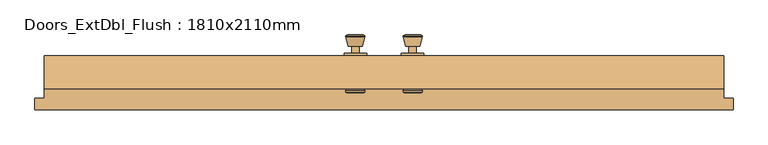
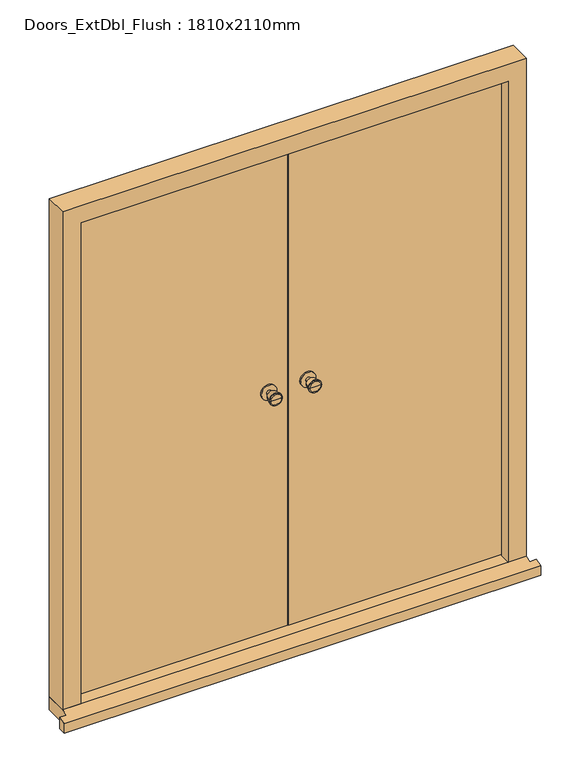
"""IFC4 building model written with IfcOpenShell, lengths in millimetres: door geometry, Doors_ExtDbl_Flush : 1810x2110mm."""

from ifc_helpers import new_model, si_unit, point, frame, frame_2d, origin, place, context, project, spatial, polyline, circle_curve, trimmed, segment, composite_curve, outline, extrude, faceted_brep, source, transform, mapped, element, save
from ifc_brep_helpers import plane_surface, cylinder_surface, revolved_surface, advanced_brep


def doors_extdbl_flush_1810x2110mm_cf8af4c5(model_context):
    return source(origin(), model_context, "Body", "SolidModel", [
        advanced_brep(
        [(-76.5, 7.5, 1050.0), (-86.5, 7.5, 1050.0), (-66.5, 7.5, 1050.0), (-96.9758676, 56.5, 1050.0), (-76.5, 56.5, 1050.0), (-56.0241324, 56.5, 1050.0), (-101.5, 54.6721319, 1050.0), (-51.5, 54.6721319, 1050.0), (-101.5, 51.2084537, 1050.0), (-51.5, 51.2084537, 1050.0), (-95.136236, 26.5, 1050.0), (-57.863764, 26.5, 1050.0), (-86.5, 26.5, 1050.0), (-66.5, 26.5, 1050.0)],
        [
            (0, 1),
            (1, 2, circle_curve(frame((-76.5, 7.5, 1050.0), z_axis=(0.0, -1.0, 0.0), x_axis=(1.0, 0.0, 0.0)), 10.0)),
            (2, 0),
            (2, 1, circle_curve(frame((-76.5, 7.5, 1050.0), z_axis=(0.0, -1.0, 0.0), x_axis=(1.0, 0.0, 0.0)), 10.0)),
            (3, 4),
            (4, 5),
            (5, 3, circle_curve(frame((-76.5, 56.5, 1050.0), z_axis=(0.0, 1.0, 0.0), x_axis=(1.0, 0.0, 0.0)), 20.4758676)),
            (3, 5, circle_curve(frame((-76.5, 56.5, 1050.0), z_axis=(0.0, 1.0, 0.0), x_axis=(1.0, 0.0, 0.0)), 20.4758676)),
            (6, 3),
            (5, 7),
            (7, 6, circle_curve(frame((-76.5, 54.6721319, 1050.0), z_axis=(0.0, 1.0, 0.0), x_axis=(1.0, 0.0, 0.0)), 25.0)),
            (6, 7, circle_curve(frame((-76.5, 54.6721319, 1050.0), z_axis=(0.0, 1.0, 0.0), x_axis=(1.0, 0.0, 0.0)), 25.0)),
            (8, 6),
            (7, 9),
            (9, 8, circle_curve(frame((-76.5, 51.2084537, 1050.0), z_axis=(0.0, 1.0, 0.0), x_axis=(1.0, 0.0, 0.0)), 25.0)),
            (8, 9, circle_curve(frame((-76.5, 51.2084537, 1050.0), z_axis=(0.0, 1.0, 0.0), x_axis=(1.0, 0.0, 0.0)), 25.0)),
            (10, 8),
            (9, 11),
            (11, 10, circle_curve(frame((-76.5, 26.5, 1050.0), z_axis=(0.0, 1.0, 0.0), x_axis=(1.0, 0.0, 0.0)), 18.636236)),
            (10, 11, circle_curve(frame((-76.5, 26.5, 1050.0), z_axis=(0.0, 1.0, 0.0), x_axis=(1.0, 0.0, 0.0)), 18.636236)),
            (12, 10),
            (11, 13),
            (13, 12, circle_curve(frame((-76.5, 26.5, 1050.0), z_axis=(0.0, 1.0, 0.0), x_axis=(1.0, 0.0, 0.0)), 10.0)),
            (12, 13, circle_curve(frame((-76.5, 26.5, 1050.0), z_axis=(0.0, 1.0, 0.0), x_axis=(1.0, 0.0, 0.0)), 10.0)),
            (1, 12),
            (13, 2),
        ],
        [
            plane_surface(frame((-76.5, 7.5, 1050.0), z_axis=(0.0, -1.0, 0.0), x_axis=(1.0, 0.0, 0.0))),
            plane_surface(frame((-76.5, 56.5, 1050.0), z_axis=(0.0, 1.0, 0.0), x_axis=(1.0, 0.0, 0.0))),
            revolved_surface(polyline([(-56.0241324, 56.5, 1050.0), (-51.5, 54.6721319, 1050.0)]), (-76.5, 7.5, 1050.0), (0.0, -1.0, 0.0)),
            cylinder_surface(frame((-76.5, 7.5, 1050.0), z_axis=(0.0, -1.0, 0.0), x_axis=(1.0, 0.0, 0.0)), 25.0),
            revolved_surface(polyline([(-51.5, 51.2084537, 1050.0), (-57.863764, 26.5, 1050.0)]), (-76.5, 7.5, 1050.0), (0.0, -1.0, 0.0)),
            plane_surface(frame((-76.5, 26.5, 1050.0), z_axis=(0.0, -1.0, 0.0), x_axis=(1.0, 0.0, 0.0))),
            cylinder_surface(frame((-76.5, 7.5, 1050.0), z_axis=(0.0, -1.0, 0.0), x_axis=(1.0, 0.0, 0.0)), 10.0),
        ],
        [
            (0, [[1, 2, 3]]),
            (0, [[-3, 4, -1]]),
            (1, [[5, 6, 7]]),
            (1, [[-6, -5, 8]]),
            (2, [[9, -7, 10, 11]]),
            (2, [[-10, -8, -9, 12]]),
            (3, [[13, -11, 14, 15]]),
            (3, [[-14, -12, -13, 16]]),
            (4, [[17, -15, 18, 19]]),
            (4, [[-18, -16, -17, 20]]),
            (5, [[21, -19, 22, 23]]),
            (5, [[-22, -20, -21, 24]]),
            (6, [[25, -23, 26, -2]]),
            (6, [[-26, -24, -25, -4]]),
        ],
    ),
        extrude(outline(composite_curve([segment(trimmed(circle_curve(frame_2d((1050.0, -76.5)), 30.0), [point((1050.0, -46.5))], [point((1050.0, -106.5))], False, "CARTESIAN"), True, "CONTINUOUS"), segment(trimmed(circle_curve(frame_2d((1050.0, -76.5)), 30.0), [point((1050.0, -106.5))], [point((1050.0, -46.5))], False, "CARTESIAN"), True, "CONTINUOUS")], self_intersect=False)), frame((0.0, 1.5, 0.0), z_axis=(0.0, 1.0, 0.0), x_axis=(0.0, 0.0, 1.0)), (0.0, 0.0, 1.0), 6.0),
        advanced_brep(
        [(-76.5, -48.5, 1050.0), (-66.5, -48.5, 1050.0), (-86.5, -48.5, 1050.0), (-96.9758676, -97.5, 1050.0), (-56.0241324, -97.5, 1050.0), (-76.5, -97.5, 1050.0), (-101.5, -95.6721319, 1050.0), (-51.5, -95.6721319, 1050.0), (-101.5, -92.2084537, 1050.0), (-51.5, -92.2084537, 1050.0), (-95.136236, -67.5, 1050.0), (-57.863764, -67.5, 1050.0), (-86.5, -67.5, 1050.0), (-66.5, -67.5, 1050.0)],
        [
            (0, 1),
            (1, 2, circle_curve(frame((-76.5, -48.5, 1050.0), z_axis=(0.0, 1.0, 0.0), x_axis=(1.0, 0.0, 0.0)), 10.0)),
            (2, 0),
            (2, 1, circle_curve(frame((-76.5, -48.5, 1050.0), z_axis=(0.0, 1.0, 0.0), x_axis=(1.0, 0.0, 0.0)), 10.0)),
            (3, 4, circle_curve(frame((-76.5, -97.5, 1050.0), z_axis=(0.0, -1.0, 0.0), x_axis=(1.0, 0.0, 0.0)), 20.4758676)),
            (4, 5),
            (5, 3),
            (4, 3, circle_curve(frame((-76.5, -97.5, 1050.0), z_axis=(0.0, -1.0, 0.0), x_axis=(1.0, 0.0, 0.0)), 20.4758676)),
            (6, 7, circle_curve(frame((-76.5, -95.6721319, 1050.0), z_axis=(0.0, -1.0, 0.0), x_axis=(1.0, 0.0, 0.0)), 25.0)),
            (7, 4),
            (3, 6),
            (7, 6, circle_curve(frame((-76.5, -95.6721319, 1050.0), z_axis=(0.0, -1.0, 0.0), x_axis=(1.0, 0.0, 0.0)), 25.0)),
            (8, 9, circle_curve(frame((-76.5, -92.2084537, 1050.0), z_axis=(0.0, -1.0, 0.0), x_axis=(1.0, 0.0, 0.0)), 25.0)),
            (9, 7),
            (6, 8),
            (9, 8, circle_curve(frame((-76.5, -92.2084537, 1050.0), z_axis=(0.0, -1.0, 0.0), x_axis=(1.0, 0.0, 0.0)), 25.0)),
            (10, 11, circle_curve(frame((-76.5, -67.5, 1050.0), z_axis=(0.0, -1.0, 0.0), x_axis=(1.0, 0.0, 0.0)), 18.636236)),
            (11, 9),
            (8, 10),
            (11, 10, circle_curve(frame((-76.5, -67.5, 1050.0), z_axis=(0.0, -1.0, 0.0), x_axis=(1.0, 0.0, 0.0)), 18.636236)),
            (12, 13, circle_curve(frame((-76.5, -67.5, 1050.0), z_axis=(0.0, -1.0, 0.0), x_axis=(1.0, 0.0, 0.0)), 10.0)),
            (13, 11),
            (10, 12),
            (13, 12, circle_curve(frame((-76.5, -67.5, 1050.0), z_axis=(0.0, -1.0, 0.0), x_axis=(1.0, 0.0, 0.0)), 10.0)),
            (1, 13),
            (12, 2),
        ],
        [
            plane_surface(frame((-76.5, -48.5, 1050.0), z_axis=(0.0, 1.0, 0.0), x_axis=(1.0, 0.0, 0.0))),
            plane_surface(frame((-76.5, -97.5, 1050.0), z_axis=(0.0, -1.0, 0.0), x_axis=(1.0, 0.0, 0.0))),
            revolved_surface(polyline([(-56.0241324, -97.5, 1050.0), (-51.5, -95.6721319, 1050.0)]), (-76.5, -48.5, 1050.0), (0.0, 1.0, 0.0)),
            cylinder_surface(frame((-76.5, -48.5, 1050.0), z_axis=(0.0, 1.0, 0.0), x_axis=(1.0, 0.0, 0.0)), 25.0),
            revolved_surface(polyline([(-51.5, -92.2084537, 1050.0), (-57.863764, -67.5, 1050.0)]), (-76.5, -48.5, 1050.0), (0.0, 1.0, 0.0)),
            plane_surface(frame((-76.5, -67.5, 1050.0), z_axis=(0.0, 1.0, 0.0), x_axis=(1.0, 0.0, 0.0))),
            cylinder_surface(frame((-76.5, -48.5, 1050.0), z_axis=(0.0, 1.0, 0.0), x_axis=(1.0, 0.0, 0.0)), 10.0),
        ],
        [
            (0, [[1, 2, 3]]),
            (0, [[-3, 4, -1]]),
            (1, [[5, 6, 7]]),
            (1, [[8, -7, -6]]),
            (2, [[9, 10, -5, 11]]),
            (2, [[12, -11, -8, -10]]),
            (3, [[13, 14, -9, 15]]),
            (3, [[16, -15, -12, -14]]),
            (4, [[17, 18, -13, 19]]),
            (4, [[20, -19, -16, -18]]),
            (5, [[21, 22, -17, 23]]),
            (5, [[24, -23, -20, -22]]),
            (6, [[-2, 25, -21, 26]]),
            (6, [[-4, -26, -24, -25]]),
        ],
    ),
        extrude(outline(composite_curve([segment(trimmed(circle_curve(frame_2d((1050.0, -76.5)), 30.0), [point((1050.0, -46.5))], [point((1050.0, -106.5))], False, "CARTESIAN"), True, "CONTINUOUS"), segment(trimmed(circle_curve(frame_2d((1050.0, -76.5)), 30.0), [point((1050.0, -106.5))], [point((1050.0, -46.5))], False, "CARTESIAN"), True, "CONTINUOUS")], self_intersect=False)), frame((0.0, -48.5, 0.0), z_axis=(0.0, 1.0, 0.0), x_axis=(0.0, 0.0, 1.0)), (0.0, 0.0, 1.0), 6.0),
        advanced_brep(
        [(76.5, 7.5, 1050.0), (66.5, 7.5, 1050.0), (86.5, 7.5, 1050.0), (96.9758676, 56.5, 1050.0), (56.0241324, 56.5, 1050.0), (76.5, 56.5, 1050.0), (101.5, 54.6721319, 1050.0), (51.5, 54.6721319, 1050.0), (101.5, 51.2084537, 1050.0), (51.5, 51.2084537, 1050.0), (95.136236, 26.5, 1050.0), (57.863764, 26.5, 1050.0), (86.5, 26.5, 1050.0), (66.5, 26.5, 1050.0)],
        [
            (0, 1),
            (1, 2, circle_curve(frame((76.5, 7.5, 1050.0), z_axis=(0.0, -1.0, 0.0), x_axis=(-1.0, 0.0, 0.0)), 10.0)),
            (2, 0),
            (2, 1, circle_curve(frame((76.5, 7.5, 1050.0), z_axis=(0.0, -1.0, 0.0), x_axis=(-1.0, 0.0, 0.0)), 10.0)),
            (3, 4, circle_curve(frame((76.5, 56.5, 1050.0), z_axis=(0.0, 1.0, 0.0), x_axis=(-1.0, 0.0, 0.0)), 20.4758676)),
            (4, 5),
            (5, 3),
            (4, 3, circle_curve(frame((76.5, 56.5, 1050.0), z_axis=(0.0, 1.0, 0.0), x_axis=(-1.0, 0.0, 0.0)), 20.4758676)),
            (6, 7, circle_curve(frame((76.5, 54.6721319, 1050.0), z_axis=(0.0, 1.0, 0.0), x_axis=(-1.0, 0.0, 0.0)), 25.0)),
            (7, 4),
            (3, 6),
            (7, 6, circle_curve(frame((76.5, 54.6721319, 1050.0), z_axis=(0.0, 1.0, 0.0), x_axis=(-1.0, 0.0, 0.0)), 25.0)),
            (8, 9, circle_curve(frame((76.5, 51.2084537, 1050.0), z_axis=(0.0, 1.0, 0.0), x_axis=(-1.0, 0.0, 0.0)), 25.0)),
            (9, 7),
            (6, 8),
            (9, 8, circle_curve(frame((76.5, 51.2084537, 1050.0), z_axis=(0.0, 1.0, 0.0), x_axis=(-1.0, 0.0, 0.0)), 25.0)),
            (10, 11, circle_curve(frame((76.5, 26.5, 1050.0), z_axis=(0.0, 1.0, 0.0), x_axis=(-1.0, 0.0, 0.0)), 18.636236)),
            (11, 9),
            (8, 10),
            (11, 10, circle_curve(frame((76.5, 26.5, 1050.0), z_axis=(0.0, 1.0, 0.0), x_axis=(-1.0, 0.0, 0.0)), 18.636236)),
            (12, 13, circle_curve(frame((76.5, 26.5, 1050.0), z_axis=(0.0, 1.0, 0.0), x_axis=(-1.0, 0.0, 0.0)), 10.0)),
            (13, 11),
            (10, 12),
            (13, 12, circle_curve(frame((76.5, 26.5, 1050.0), z_axis=(0.0, 1.0, 0.0), x_axis=(-1.0, 0.0, 0.0)), 10.0)),
            (1, 13),
            (12, 2),
        ],
        [
            plane_surface(frame((76.5, 7.5, 1050.0), z_axis=(0.0, -1.0, 0.0), x_axis=(-1.0, 0.0, 0.0))),
            plane_surface(frame((76.5, 56.5, 1050.0), z_axis=(0.0, 1.0, 0.0), x_axis=(-1.0, 0.0, 0.0))),
            revolved_surface(polyline([(56.0241324, 56.5, 1050.0), (51.5, 54.6721319, 1050.0)]), (76.5, 7.5, 1050.0), (0.0, -1.0, 0.0)),
            cylinder_surface(frame((76.5, 7.5, 1050.0), z_axis=(0.0, -1.0, 0.0), x_axis=(-1.0, 0.0, 0.0)), 25.0),
            revolved_surface(polyline([(51.5, 51.2084537, 1050.0), (57.863764, 26.5, 1050.0)]), (76.5, 7.5, 1050.0), (0.0, -1.0, 0.0)),
            plane_surface(frame((76.5, 26.5, 1050.0), z_axis=(0.0, -1.0, 0.0), x_axis=(-1.0, 0.0, 0.0))),
            cylinder_surface(frame((76.5, 7.5, 1050.0), z_axis=(0.0, -1.0, 0.0), x_axis=(-1.0, 0.0, 0.0)), 10.0),
        ],
        [
            (0, [[1, 2, 3]]),
            (0, [[-3, 4, -1]]),
            (1, [[5, 6, 7]]),
            (1, [[8, -7, -6]]),
            (2, [[9, 10, -5, 11]]),
            (2, [[12, -11, -8, -10]]),
            (3, [[13, 14, -9, 15]]),
            (3, [[16, -15, -12, -14]]),
            (4, [[17, 18, -13, 19]]),
            (4, [[20, -19, -16, -18]]),
            (5, [[21, 22, -17, 23]]),
            (5, [[24, -23, -20, -22]]),
            (6, [[-2, 25, -21, 26]]),
            (6, [[-4, -26, -24, -25]]),
        ],
    ),
        extrude(outline(composite_curve([segment(trimmed(circle_curve(frame_2d((1050.0, 76.5)), 30.0), [point((1050.0, 46.5))], [point((1050.0, 106.5))], False, "CARTESIAN"), True, "CONTINUOUS"), segment(trimmed(circle_curve(frame_2d((1050.0, 76.5)), 30.0), [point((1050.0, 106.5))], [point((1050.0, 46.5))], False, "CARTESIAN"), True, "CONTINUOUS")], self_intersect=False)), frame((0.0, 1.5, 0.0), z_axis=(0.0, 1.0, 0.0), x_axis=(0.0, 0.0, 1.0)), (0.0, 0.0, 1.0), 6.0),
        advanced_brep(
        [(76.5, -48.5, 1050.0), (86.5, -48.5, 1050.0), (66.5, -48.5, 1050.0), (96.9758676, -97.5, 1050.0), (76.5, -97.5, 1050.0), (56.0241324, -97.5, 1050.0), (101.5, -95.6721319, 1050.0), (51.5, -95.6721319, 1050.0), (101.5, -92.2084537, 1050.0), (51.5, -92.2084537, 1050.0), (95.136236, -67.5, 1050.0), (57.863764, -67.5, 1050.0), (86.5, -67.5, 1050.0), (66.5, -67.5, 1050.0)],
        [
            (0, 1),
            (1, 2, circle_curve(frame((76.5, -48.5, 1050.0), z_axis=(0.0, 1.0, 0.0), x_axis=(-1.0, 0.0, 0.0)), 10.0)),
            (2, 0),
            (2, 1, circle_curve(frame((76.5, -48.5, 1050.0), z_axis=(0.0, 1.0, 0.0), x_axis=(-1.0, 0.0, 0.0)), 10.0)),
            (3, 4),
            (4, 5),
            (5, 3, circle_curve(frame((76.5, -97.5, 1050.0), z_axis=(0.0, -1.0, 0.0), x_axis=(-1.0, 0.0, 0.0)), 20.4758676)),
            (3, 5, circle_curve(frame((76.5, -97.5, 1050.0), z_axis=(0.0, -1.0, 0.0), x_axis=(-1.0, 0.0, 0.0)), 20.4758676)),
            (6, 3),
            (5, 7),
            (7, 6, circle_curve(frame((76.5, -95.6721319, 1050.0), z_axis=(0.0, -1.0, 0.0), x_axis=(-1.0, 0.0, 0.0)), 25.0)),
            (6, 7, circle_curve(frame((76.5, -95.6721319, 1050.0), z_axis=(0.0, -1.0, 0.0), x_axis=(-1.0, 0.0, 0.0)), 25.0)),
            (8, 6),
            (7, 9),
            (9, 8, circle_curve(frame((76.5, -92.2084537, 1050.0), z_axis=(0.0, -1.0, 0.0), x_axis=(-1.0, 0.0, 0.0)), 25.0)),
            (8, 9, circle_curve(frame((76.5, -92.2084537, 1050.0), z_axis=(0.0, -1.0, 0.0), x_axis=(-1.0, 0.0, 0.0)), 25.0)),
            (10, 8),
            (9, 11),
            (11, 10, circle_curve(frame((76.5, -67.5, 1050.0), z_axis=(0.0, -1.0, 0.0), x_axis=(-1.0, 0.0, 0.0)), 18.636236)),
            (10, 11, circle_curve(frame((76.5, -67.5, 1050.0), z_axis=(0.0, -1.0, 0.0), x_axis=(-1.0, 0.0, 0.0)), 18.636236)),
            (12, 10),
            (11, 13),
            (13, 12, circle_curve(frame((76.5, -67.5, 1050.0), z_axis=(0.0, -1.0, 0.0), x_axis=(-1.0, 0.0, 0.0)), 10.0)),
            (12, 13, circle_curve(frame((76.5, -67.5, 1050.0), z_axis=(0.0, -1.0, 0.0), x_axis=(-1.0, 0.0, 0.0)), 10.0)),
            (1, 12),
            (13, 2),
        ],
        [
            plane_surface(frame((76.5, -48.5, 1050.0), z_axis=(0.0, 1.0, 0.0), x_axis=(-1.0, 0.0, 0.0))),
            plane_surface(frame((76.5, -97.5, 1050.0), z_axis=(0.0, -1.0, 0.0), x_axis=(-1.0, 0.0, 0.0))),
            revolved_surface(polyline([(56.0241324, -97.5, 1050.0), (51.5, -95.6721319, 1050.0)]), (76.5, -48.5, 1050.0), (0.0, 1.0, 0.0)),
            cylinder_surface(frame((76.5, -48.5, 1050.0), z_axis=(0.0, 1.0, 0.0), x_axis=(-1.0, 0.0, 0.0)), 25.0),
            revolved_surface(polyline([(51.5, -92.2084537, 1050.0), (57.863764, -67.5, 1050.0)]), (76.5, -48.5, 1050.0), (0.0, 1.0, 0.0)),
            plane_surface(frame((76.5, -67.5, 1050.0), z_axis=(0.0, 1.0, 0.0), x_axis=(-1.0, 0.0, 0.0))),
            cylinder_surface(frame((76.5, -48.5, 1050.0), z_axis=(0.0, 1.0, 0.0), x_axis=(-1.0, 0.0, 0.0)), 10.0),
        ],
        [
            (0, [[1, 2, 3]]),
            (0, [[-3, 4, -1]]),
            (1, [[5, 6, 7]]),
            (1, [[-6, -5, 8]]),
            (2, [[9, -7, 10, 11]]),
            (2, [[-10, -8, -9, 12]]),
            (3, [[13, -11, 14, 15]]),
            (3, [[-14, -12, -13, 16]]),
            (4, [[17, -15, 18, 19]]),
            (4, [[-18, -16, -17, 20]]),
            (5, [[21, -19, 22, 23]]),
            (5, [[-22, -20, -21, 24]]),
            (6, [[25, -23, 26, -2]]),
            (6, [[-26, -24, -25, -4]]),
        ],
    ),
        extrude(outline(composite_curve([segment(trimmed(circle_curve(frame_2d((1050.0, 76.5)), 30.0), [point((1050.0, 46.5))], [point((1050.0, 106.5))], False, "CARTESIAN"), True, "CONTINUOUS"), segment(trimmed(circle_curve(frame_2d((1050.0, 76.5)), 30.0), [point((1050.0, 106.5))], [point((1050.0, 46.5))], False, "CARTESIAN"), True, "CONTINUOUS")], self_intersect=False)), frame((0.0, -48.5, 0.0), z_axis=(0.0, 1.0, 0.0), x_axis=(0.0, 0.0, 1.0)), (0.0, 0.0, 1.0), 6.0),
        faceted_brep([(834.5, -87.5, 54.5), (834.5, -45.5, 54.5), (856.5, -45.5, 54.5), (856.5, 1.5, 54.5), (905.0, 1.5, 54.5), (905.0, -87.5, 54.5), (905.0, -87.5, 2110.0), (-905.0, -87.5, 2110.0), (-905.0, -87.5, 54.5), (-834.5, -87.5, 54.5), (-834.5, -87.5, 2039.5), (834.5, -87.5, 2039.5), (905.0, 1.5, 2110.0), (856.5, 1.5, 2061.5), (-856.5, 1.5, 2061.5), (-856.5, 1.5, 54.5), (-905.0, 1.5, 54.5), (-905.0, 1.5, 2110.0), (856.5, -45.5, 2061.5), (834.5, -45.5, 2039.5), (-834.5, -45.5, 2039.5), (-834.5, -45.5, 54.5), (-856.5, -45.5, 54.5), (-856.5, -45.5, 2061.5)], [[[0, 1, 2, 3, 4, 5]], [[5, 6, 7, 8, 9, 10, 11, 0]], [[4, 12, 6, 5]], [[3, 13, 14, 15, 16, 17, 12, 4]], [[2, 18, 13, 3]], [[1, 19, 20, 21, 22, 23, 18, 2]], [[0, 11, 19, 1]], [[12, 17, 7, 6]], [[18, 23, 14, 13]], [[11, 10, 20, 19]], [[9, 8, 16, 15, 22, 21]], [[17, 16, 8, 7]], [[23, 22, 15, 14]], [[10, 9, 21, 20]]]),
        faceted_brep([(930.0, -142.5, 0.0), (930.0, -112.5, 0.0), (930.0, -112.5, 47.2703282), (930.0, -142.5, 38.5947221), (-930.0, -142.5, 38.5947221), (-930.0, -112.5, 47.2703282), (-930.0, -112.5, 0.0), (-930.0, -142.5, 0.0), (-905.0, -112.5, 0.0), (-905.0, 1.5, 0.0), (905.0, 1.5, 0.0), (905.0, -112.5, 0.0), (905.0, -112.5, 47.2703282), (905.0, -87.5, 54.5), (-905.0, -87.5, 54.5), (-905.0, -112.5, 47.2703282), (905.0, 1.5, 54.5), (-905.0, 1.5, 54.5)], [[[0, 1, 2, 3]], [[4, 5, 6, 7]], [[7, 6, 8, 9, 10, 11, 1, 0]], [[3, 4, 7, 0]], [[3, 2, 12, 13, 14, 15, 5, 4]], [[14, 13, 16, 17]], [[17, 16, 10, 9]], [[15, 14, 17, 9, 8]], [[8, 6, 5, 15]], [[11, 10, 16, 13, 12]], [[12, 2, 1, 11]]]),
        extrude(outline(polyline([(853.5, 1.5), (853.5, -42.5), (1.5, -42.5), (1.5, 1.5), (853.5, 1.5)])), frame((0.0, 0.0, 58.5), z_axis=(0.0, 0.0, 1.0), x_axis=(1.0, 0.0, 0.0)), (0.0, 0.0, 1.0), 2000.0),
        extrude(outline(polyline([(-1.5, 1.5), (-1.5, -42.5), (-853.5, -42.5), (-853.5, 1.5), (-1.5, 1.5)])), frame((0.0, 0.0, 58.5), z_axis=(0.0, 0.0, 1.0), x_axis=(1.0, 0.0, 0.0)), (0.0, 0.0, 1.0), 2000.0),
    ])


if __name__ == "__main__":
    model = new_model("IFC4")
    model_context = context("Model", 3, world=origin())
    ifc_project = project(units=[si_unit("LENGTHUNIT", "METRE", prefix="MILLI")], contexts=[model_context])
    site = spatial("IfcSite", under=ifc_project)
    building = spatial("IfcBuilding", under=site)
    placement = place(None, origin())
    doors_extdbl_flush_1810x2110mm_shape = doors_extdbl_flush_1810x2110mm_cf8af4c5(model_context)
    element("IfcDoor", 1, ObjectType="Doors_ExtDbl_Flush : 1810x2110mm", at=placement, inside=building, context=model_context, shape_type="MappedRepresentation", body=[
        mapped(doors_extdbl_flush_1810x2110mm_shape, transform((0.0, 0.0, 0.0), x_axis=(1.0, 0.0, 0.0), y_axis=(0.0, 1.0, 0.0), z_axis=(0.0, 0.0, 1.0))),
    ])
    save(model, "model.ifc")

# Revit data of these elements
# Type "Doors_ExtDbl_Flush : 1810x2110mm"
#   Type Mark = "44"
#   Type Comments = "External Double"
#   Operation = "DoubleDoorSingleSwing"
#   Keynote = "L20"
#   Analytic Construction = "Metal"
#   Wrap Layers (Ext) from Ext = 102.5 mm
#   Wrap Layers (Int) from Ext = 177.5 mm
#   Thickness = 44 mm
#   Rough Width = 1810 mm
#   Rough Height = 2110 mm
#   O/A Frame Width = 64 mm
#   Heat Transfer Coefficient (U) = 3.7021 W/(m²·K)
#   Handle Z Distance = 1050 mm
#   FrameWidth = 42 mm
#   FrameOffset - External = 25 mm
#   FrameDepth = 89 mm
#   Door Panel Width = 852 mm
#   Door Panel Thickness = 44 mm
#   Door Panel Height = 2000 mm
#   Cill Thickness = 54.5 mm
#   Cill Projection = 30 mm
#   Handle X Distance = 75 mm
#   Height = 2110 mm
#   Structural Tolerance = 6.5 mm
#   Tolerance = 3 mm
#   Undercut = 4 mm
#   Width = 1810 mm
#   Cill Extension = 25 mm
#   Cavity Closer Width = 50 mm
#   Cavity Closer Offset from Ext = 102.5 mm
#   Cavity Closer Depth = 85 mm
#   Define Thermal Properties by = 0
#   Vis - Ironmongery = yes
#   Vis - Cavity Closers = yes
#   Function = 1
#   Material Door = Door - Panel
#   Material Frame = Door - Frame/Mullion
#   Material Ironmongery = Door - Handle
#   Visual Light Transmittance = 0
#   Thermal Resistance (R) = 0
#   Solar Heat Gain Coefficient = 0
#   Wall Closure = (empty or 0)
# Element 1 (IfcDoor, "Doors_ExtDbl_Flush : 1810x2110mm")
#   Materials on its faces: "Door - Handle", "Door - Frame/Mullion", "Door - Panel"
# Materials
#   "Door - Panel": class "Wood", colour RGB 210 159 95, transparency 0, Keynote = "L20", Cost = 0
#   "Door - Frame/Mullion": class "Wood", colour RGB 212 179 113, transparency 0, Keynote = "L20", Cost = 0
#   "Door - Handle": colour RGB 0 0 0, transparency 0, Keynote = "P21", Cost = 0
